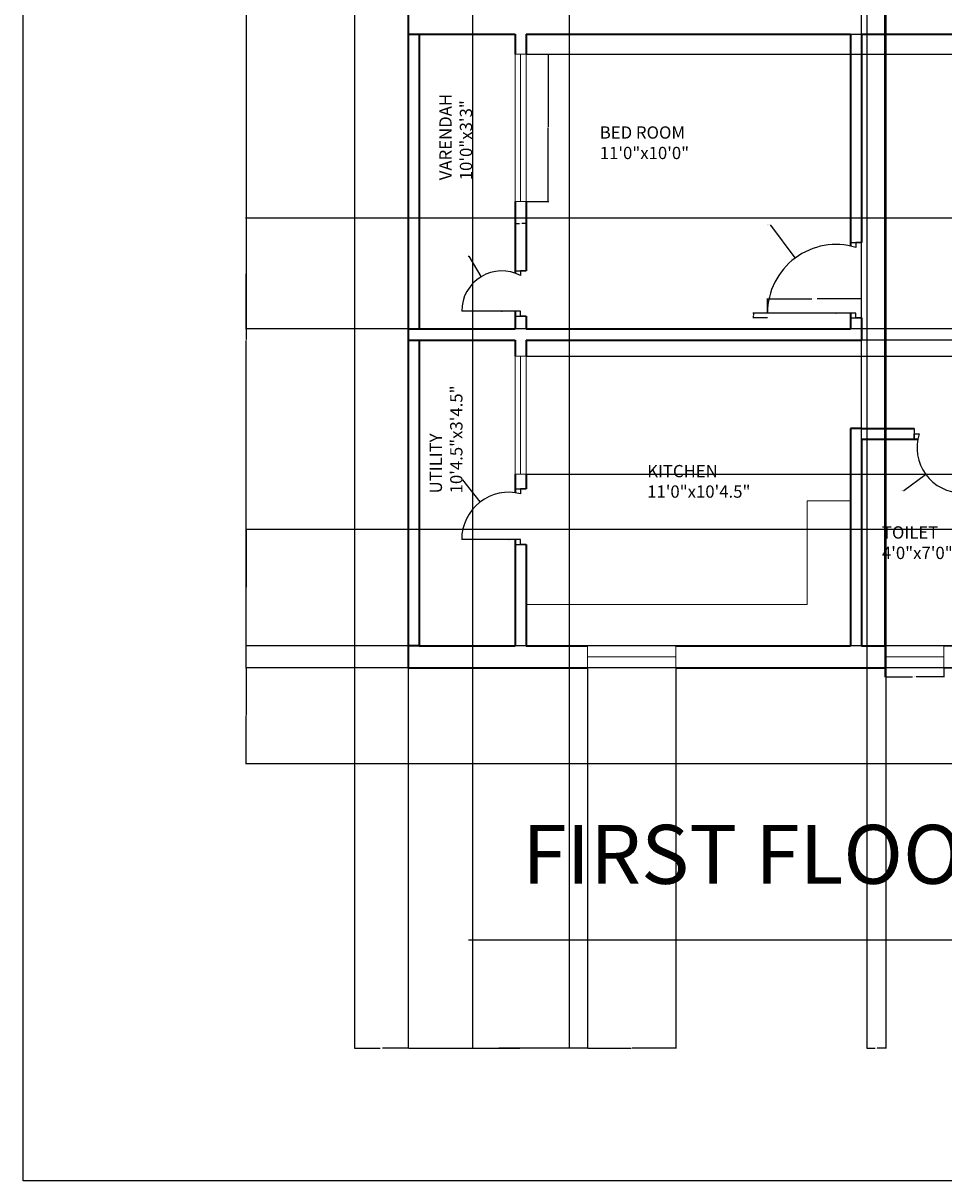
# Model space of a CAD drawing. Units: inches. Extents: x 1870 to 2611, y 1432 to 2511.
# Tile 1 of 5: x 1870 to 2245, y 1432 to 1903. Entities that reach past the tile are written whole.
import ezdxf

# ---------------------------------------------------------------- set-up
doc = ezdxf.new("R2010")
doc.units = ezdxf.units.IN
for name, color, linetype, lineweight in [('A-ANNO-DIMS', 2, 'Continuous', 18), ('A-ANNO-TTLB', 7, 'Continuous', 25), ('A-AREA-IDEN', 7, 'Continuous', 18), ('A-DOOR', 31, 'Continuous', 25), ('A-FLOR-FIXT', 8, 'Continuous', 18), ('A-GLAZ', 201, 'Continuous', 18), ('A-WALL', 7, 'Continuous', 35)]:
    doc.layers.add(name, color=color, linetype=linetype, lineweight=lineweight)
doc.styles.get("Standard").update_dxf_attribs({"font": 'arial.ttf'})
doc.dimstyles.get("Standard").update_dxf_attribs({"dimtxt": 0.18, "dimasz": 0.18, "dimexe": 0.18, "dimexo": 0.0625, "dimgap": 0.09, "dimtad": 0, "dimtih": 1, "dimtoh": 1, "dimdec": 4, "dimzin": 0, "dimdsep": 46, "dimtxsty": 'Standard', "dimcen": 0.09, "dimadec": 0, "dimazin": 0, "dimtfac": 1, "dimtdec": 4, "dimtofl": 0, "dimtmove": 0, "dimatfit": 3, "dimfxl": 1, "dimtolj": 1, "dimtzin": 0, "dimarcsym": 0})

# ---------------------------------------------------------------- blocks, each defined once
blk = doc.blocks.new('DOOR-LEAF-36-JAMB-4P5')
for p, q in [((36, 2), (0, 2)), ((33.75, 0), (38.25, 0)), ((36, 0), (36, 2)), ((38.25, 0), (36, 0))]:
    blk.add_line(p, q)
blk = doc.blocks.new('DOOR-LEAF-24-JAMB-4P5')
for p, q in [((2, 2.25), (2, 26.25)), ((0, 4.5), (0, 0)), ((0, 0), (0, 2.25)), ((0, 2.25), (2, 2.25))]:
    blk.add_line(p, q)
blk = doc.blocks.new('WIN-24-FRAME-9')
for p, q in [((0, 9), (0, 0)), ((24, 9), (0, 9)), ((24, 4.5), (24, 9)), ((24, 9), (24, 0)), ((0, 0), (0, 4.5)), ((0, 4.5), (24, 4.5)), ((0, 0), (24, 0))]:
    blk.add_line(p, q)
blk = doc.blocks.new('WIN-60-FRAME-4P5')
for p, q in [((0, 60), (4.5, 60)), ((0, 60), (0, 0)), ((4.5, 60), (2.25, 60)), ((2.25, 60), (2.25, 0)), ((4.5, 60), (4.5, 0)), ((2.25, 0), (0, 0)), ((0, 0), (4.5, 0))]:
    blk.add_line(p, q)
blk = doc.blocks.new('*D13')
at = {"layer": 'A-ANNO-DIMS', "color": 0, "lineweight": -2, "transparency": 16777216}
for p, q in [((2172.77, 1784.92), (2172.77, 1790.78)), ((2172.95, 1790.6), (2190.84, 1790.6)), ((2210.84, 1790.6), (2192.95, 1790.6)), ((2211.02, 1784.92), (2211.02, 1790.78))]:
    blk.add_line(p, q, dxfattribs=at)
at = {"layer": 'A-ANNO-DIMS', "color": 0, "transparency": 16777216}
for points in [[(2172.95, 1790.63), (2172.95, 1790.57), (2172.77, 1790.6)], [(2210.84, 1790.63), (2210.84, 1790.57), (2211.02, 1790.6)]]:
    blk.add_solid(points, dxfattribs=at)
at = {"layer": 'Defpoints', "color": 0, "transparency": 16777216}
for p in [(2211.02, 1790.6), (2172.77, 1784.86), (2211.02, 1784.86)]:
    blk.add_point(p, dxfattribs=at)
at = {"layer": 'A-ANNO-DIMS', "color": 0, "transparency": 16777216, "insert": (2191.89, 1790.6), "char_height": 0.18, "attachment_point": 5}
blk.add_mtext('\\A1;DOOR B 38 TYP.', dxfattribs=at)
blk = doc.blocks.new('*D14')
at = {"layer": 'A-ANNO-DIMS', "color": 0, "lineweight": -2, "transparency": 16777216}
for p, q in [((2172.71, 1784.86), (2166.85, 1784.86)), ((2172.71, 1782.86), (2166.85, 1782.86)), ((2167.03, 1784.68), (2167.03, 1784.04)), ((2167.03, 1783.04), (2167.03, 1783.68))]:
    blk.add_line(p, q, dxfattribs=at)
at = {"layer": 'A-ANNO-DIMS', "color": 0, "transparency": 16777216}
for points in [[(2167, 1784.68), (2167.06, 1784.68), (2167.03, 1784.86)], [(2167, 1783.04), (2167.06, 1783.04), (2167.03, 1782.86)]]:
    blk.add_solid(points, dxfattribs=at)
at = {"layer": 'Defpoints', "color": 0, "transparency": 16777216}
for p in [(2167.03, 1784.86), (2172.77, 1784.86), (2172.77, 1782.86)]:
    blk.add_point(p, dxfattribs=at)
at = {"layer": 'A-ANNO-DIMS', "color": 0, "transparency": 16777216, "insert": (2167.03, 1783.86), "char_height": 0.18, "attachment_point": 5}
blk.add_mtext('\\A1;2 TYP.', dxfattribs=at)
blk = doc.blocks.new('*D15')
at = {"layer": 'A-ANNO-DIMS', "color": 0, "lineweight": -2, "transparency": 16777216}
for p, q in [((2074.58, 1890.28), (2083.7, 1890.28)), ((2083.52, 1890.1), (2083.52, 1860.46)), ((2083.52, 1830.46), (2083.52, 1860.1)), ((2074.58, 1830.28), (2083.7, 1830.28))]:
    blk.add_line(p, q, dxfattribs=at)
at = {"layer": 'A-ANNO-DIMS', "color": 0, "transparency": 16777216}
for points in [[(2083.49, 1890.1), (2083.55, 1890.1), (2083.52, 1890.28)], [(2083.49, 1830.46), (2083.55, 1830.46), (2083.52, 1830.28)]]:
    blk.add_solid(points, dxfattribs=at)
at = {"layer": 'Defpoints', "color": 0, "transparency": 16777216}
for p in [(2074.52, 1890.28), (2074.52, 1830.28), (2083.52, 1830.28)]:
    blk.add_point(p, dxfattribs=at)
at = {"layer": 'A-ANNO-DIMS', "color": 0, "transparency": 16777216, "insert": (2083.52, 1860.28), "char_height": 0.18, "attachment_point": 5}
blk.add_mtext('\\A1;W2 60 TYP.', dxfattribs=at)
blk = doc.blocks.new('*D16')
at = {"layer": 'A-ANNO-DIMS', "color": 0, "lineweight": -2, "transparency": 16777216}
for p, q in [((2070.02, 1830.22), (2070.02, 1821.1)), ((2074.52, 1830.22), (2074.52, 1821.1)), ((2070.2, 1821.28), (2071.81, 1821.28)), ((2074.34, 1821.28), (2072.73, 1821.28))]:
    blk.add_line(p, q, dxfattribs=at)
at = {"layer": 'A-ANNO-DIMS', "color": 0, "transparency": 16777216}
for points in [[(2070.2, 1821.31), (2070.2, 1821.25), (2070.02, 1821.28)], [(2074.34, 1821.31), (2074.34, 1821.25), (2074.52, 1821.28)]]:
    blk.add_solid(points, dxfattribs=at)
at = {"layer": 'Defpoints', "color": 0, "transparency": 16777216}
for p in [(2070.02, 1830.28), (2074.52, 1830.28), (2070.02, 1821.28)]:
    blk.add_point(p, dxfattribs=at)
at = {"layer": 'A-ANNO-DIMS', "color": 0, "transparency": 16777216, "insert": (2072.27, 1821.28), "char_height": 0.18, "attachment_point": 5}
blk.add_mtext('\\A1;5 TYP.', dxfattribs=at)
blk = doc.blocks.new('*D17')
at = {"layer": 'A-ANNO-DIMS', "color": 0, "lineweight": -2, "transparency": 16777216}
for p, q in [((2220.56, 1640.3), (2220.56, 1636.59)), ((2244.56, 1640.3), (2244.56, 1636.59)), ((2220.74, 1636.77), (2231.8, 1636.77)), ((2244.38, 1636.77), (2233.31, 1636.77))]:
    blk.add_line(p, q, dxfattribs=at)
at = {"layer": 'A-ANNO-DIMS', "color": 0, "transparency": 16777216}
for points in [[(2220.74, 1636.8), (2220.74, 1636.74), (2220.56, 1636.77)], [(2244.38, 1636.8), (2244.38, 1636.74), (2244.56, 1636.77)]]:
    blk.add_solid(points, dxfattribs=at)
at = {"layer": 'Defpoints', "color": 0, "transparency": 16777216}
for p in [(2220.56, 1640.37), (2244.56, 1640.37), (2220.56, 1636.77)]:
    blk.add_point(p, dxfattribs=at)
at = {"layer": 'A-ANNO-DIMS', "color": 0, "transparency": 16777216, "insert": (2232.56, 1636.77), "char_height": 0.18, "attachment_point": 5}
blk.add_mtext('\\A1;W3 24 TYP.', dxfattribs=at)
blk = doc.blocks.new('*D18')
at = {"layer": 'A-ANNO-DIMS', "color": 0, "lineweight": -2, "transparency": 16777216}
for p, q in [((2244.62, 1649.37), (2248.34, 1649.37)), ((2248.16, 1649.19), (2248.16, 1645.05)), ((2244.62, 1640.37), (2248.34, 1640.37)), ((2248.16, 1640.55), (2248.16, 1644.69))]:
    blk.add_line(p, q, dxfattribs=at)
at = {"layer": 'A-ANNO-DIMS', "color": 0, "transparency": 16777216}
for points in [[(2248.13, 1649.19), (2248.19, 1649.19), (2248.16, 1649.37)], [(2248.13, 1640.55), (2248.19, 1640.55), (2248.16, 1640.37)]]:
    blk.add_solid(points, dxfattribs=at)
at = {"layer": 'Defpoints', "color": 0, "transparency": 16777216}
for p in [(2244.56, 1649.37), (2244.56, 1640.37), (2248.16, 1640.37)]:
    blk.add_point(p, dxfattribs=at)
at = {"layer": 'A-ANNO-DIMS', "color": 0, "transparency": 16777216, "insert": (2248.16, 1644.87), "char_height": 0.18, "attachment_point": 5}
blk.add_mtext('\\A1;9 TYP.', dxfattribs=at)
blk = doc.blocks.new('*D29')
at = {"layer": 'A-ANNO-DIMS', "color": 0, "lineweight": -2, "transparency": 16777216}
for p, q in [((2026.46, 1907.37), (1960.31, 1907.37)), ((1960.49, 1907.19), (1960.49, 1774.05)), ((1960.49, 1640.55), (1960.49, 1773.69)), ((2026.46, 1640.37), (1960.31, 1640.37))]:
    blk.add_line(p, q, dxfattribs=at)
at = {"layer": 'A-ANNO-DIMS', "color": 0, "transparency": 16777216}
for points in [[(1960.46, 1907.19), (1960.52, 1907.19), (1960.49, 1907.37)], [(1960.46, 1640.55), (1960.52, 1640.55), (1960.49, 1640.37)]]:
    blk.add_solid(points, dxfattribs=at)
at = {"layer": 'Defpoints', "color": 0, "transparency": 16777216}
for p in [(2026.52, 1907.37), (1960.49, 1640.37), (2026.52, 1640.37)]:
    blk.add_point(p, dxfattribs=at)
at = {"layer": 'A-ANNO-DIMS', "color": 0, "transparency": 16777216, "insert": (1960.49, 1773.87), "char_height": 0.18, "attachment_point": 5}
blk.add_mtext('\\A1;267', dxfattribs=at)
blk = doc.blocks.new('*D30')
at = {"layer": 'A-ANNO-DIMS', "color": 0, "lineweight": -2, "transparency": 16777216}
for p, q in [((2004.64, 2027.3), (2004.64, 1485.35)), ((2026.52, 2027.3), (2026.52, 1485.35)), ((2004.82, 1485.53), (2015.11, 1485.53)), ((2026.34, 1485.53), (2016.04, 1485.53))]:
    blk.add_line(p, q, dxfattribs=at)
at = {"layer": 'A-ANNO-DIMS', "color": 0, "transparency": 16777216}
for points in [[(2004.82, 1485.56), (2004.82, 1485.5), (2004.64, 1485.53)], [(2026.34, 1485.56), (2026.34, 1485.5), (2026.52, 1485.53)]]:
    blk.add_solid(points, dxfattribs=at)
at = {"layer": 'Defpoints', "color": 0, "transparency": 16777216}
for p in [(2004.64, 2027.37), (2026.52, 2027.37), (2026.52, 1485.53)]:
    blk.add_point(p, dxfattribs=at)
at = {"layer": 'A-ANNO-DIMS', "color": 0, "transparency": 16777216, "insert": (2015.58, 1485.53), "char_height": 0.18, "attachment_point": 5}
blk.add_mtext('\\A1;21.882', dxfattribs=at)
blk = doc.blocks.new('*D32')
at = {"layer": 'A-ANNO-DIMS', "color": 0, "lineweight": -2, "transparency": 16777216}
for p, q in [((2311.46, 1640.37), (1960.31, 1640.37)), ((1960.49, 1640.19), (1960.49, 1621.05)), ((1960.49, 1601.54), (1960.49, 1620.68)), ((2311.46, 1601.36), (1960.31, 1601.36))]:
    blk.add_line(p, q, dxfattribs=at)
at = {"layer": 'A-ANNO-DIMS', "color": 0, "transparency": 16777216}
for points in [[(1960.46, 1640.19), (1960.52, 1640.19), (1960.49, 1640.37)], [(1960.46, 1601.54), (1960.52, 1601.54), (1960.49, 1601.36)]]:
    blk.add_solid(points, dxfattribs=at)
at = {"layer": 'Defpoints', "color": 0, "transparency": 16777216}
for p in [(1960.49, 1640.37), (2311.52, 1640.37), (2311.52, 1601.36)]:
    blk.add_point(p, dxfattribs=at)
at = {"layer": 'A-ANNO-DIMS', "color": 0, "transparency": 16777216, "insert": (1960.49, 1620.86), "char_height": 0.18, "attachment_point": 5}
blk.add_mtext('\\A1;39.01', dxfattribs=at)
blk = doc.blocks.new('*D39')
at = {"layer": 'A-ANNO-DIMS', "color": 0, "lineweight": -2, "transparency": 16777216}
for p, q in [((2052.64, 2396.3), (2052.64, 1485.35)), ((2092.09, 2396.3), (2092.09, 1485.35)), ((2052.82, 1485.53), (2071.97, 1485.53)), ((2091.91, 1485.53), (2072.76, 1485.53))]:
    blk.add_line(p, q, dxfattribs=at)
at = {"layer": 'A-ANNO-DIMS', "color": 0, "transparency": 16777216}
for points in [[(2052.82, 1485.56), (2052.82, 1485.5), (2052.64, 1485.53)], [(2091.91, 1485.56), (2091.91, 1485.5), (2092.09, 1485.53)]]:
    blk.add_solid(points, dxfattribs=at)
at = {"layer": 'Defpoints', "color": 0, "transparency": 16777216}
for p in [(2052.64, 2396.37), (2092.09, 2396.37), (2092.09, 1485.53)]:
    blk.add_point(p, dxfattribs=at)
at = {"layer": 'A-ANNO-DIMS', "color": 0, "transparency": 16777216, "insert": (2072.36, 1485.53), "char_height": 0.18, "attachment_point": 5}
blk.add_mtext('\\A1;39.45', dxfattribs=at)
blk = doc.blocks.new('*D40')
at = {"layer": 'A-ANNO-DIMS', "color": 0, "lineweight": -2, "transparency": 16777216}
for p, q in [((2213.14, 2396.3), (2213.14, 1485.35)), ((2220.9, 2396.3), (2220.9, 1485.35)), ((2213.32, 1485.53), (2216.63, 1485.53)), ((2220.72, 1485.53), (2217.41, 1485.53))]:
    blk.add_line(p, q, dxfattribs=at)
at = {"layer": 'A-ANNO-DIMS', "color": 0, "transparency": 16777216}
for points in [[(2213.32, 1485.56), (2213.32, 1485.5), (2213.14, 1485.53)], [(2220.72, 1485.56), (2220.72, 1485.5), (2220.9, 1485.53)]]:
    blk.add_solid(points, dxfattribs=at)
at = {"layer": 'Defpoints', "color": 0, "transparency": 16777216}
for p in [(2213.14, 2396.37), (2220.9, 2396.37), (2220.9, 1485.53)]:
    blk.add_point(p, dxfattribs=at)
at = {"layer": 'A-ANNO-DIMS', "color": 0, "transparency": 16777216, "insert": (2217.02, 1485.53), "char_height": 0.18, "attachment_point": 5}
blk.add_mtext('\\A1;7.766', dxfattribs=at)
blk = doc.blocks.new('*D43')
at = {"layer": 'A-ANNO-DIMS', "color": 0, "lineweight": -2, "transparency": 16777216}
for p, q in [((2099.45, 1640.3), (2099.45, 1485.35)), ((2135.45, 1640.3), (2135.45, 1485.35)), ((2099.63, 1485.53), (2117.23, 1485.53)), ((2135.27, 1485.53), (2117.67, 1485.53))]:
    blk.add_line(p, q, dxfattribs=at)
at = {"layer": 'A-ANNO-DIMS', "color": 0, "transparency": 16777216}
for points in [[(2099.63, 1485.56), (2099.63, 1485.5), (2099.45, 1485.53)], [(2135.27, 1485.56), (2135.27, 1485.5), (2135.45, 1485.53)]]:
    blk.add_solid(points, dxfattribs=at)
at = {"layer": 'Defpoints', "color": 0, "transparency": 16777216}
for p in [(2099.45, 1640.37), (2135.45, 1640.37), (2135.45, 1485.53)]:
    blk.add_point(p, dxfattribs=at)
at = {"layer": 'A-ANNO-DIMS', "color": 0, "transparency": 16777216, "insert": (2117.45, 1485.53), "char_height": 0.18, "attachment_point": 5}
blk.add_mtext('\\A1;36', dxfattribs=at)
blk = doc.blocks.new('*D44')
at = {"layer": 'A-ANNO-DIMS', "color": 0, "lineweight": -2, "transparency": 16777216}
for p, q in [((2026.52, 1640.3), (2026.52, 1485.35)), ((2099.45, 1640.3), (2099.45, 1485.35)), ((2026.7, 1485.53), (2062.59, 1485.53)), ((2099.27, 1485.53), (2063.38, 1485.53))]:
    blk.add_line(p, q, dxfattribs=at)
at = {"layer": 'A-ANNO-DIMS', "color": 0, "transparency": 16777216}
for points in [[(2026.7, 1485.56), (2026.7, 1485.5), (2026.52, 1485.53)], [(2099.27, 1485.56), (2099.27, 1485.5), (2099.45, 1485.53)]]:
    blk.add_solid(points, dxfattribs=at)
at = {"layer": 'Defpoints', "color": 0, "transparency": 16777216}
for p in [(2026.52, 1640.37), (2099.45, 1640.37), (2099.45, 1485.53)]:
    blk.add_point(p, dxfattribs=at)
at = {"layer": 'A-ANNO-DIMS', "color": 0, "transparency": 16777216, "insert": (2062.99, 1485.53), "char_height": 0.18, "attachment_point": 5}
blk.add_mtext('\\A1;72.93', dxfattribs=at)
blk = doc.blocks.new('*D45')
at = {"layer": 'A-ANNO-DIMS', "color": 0, "lineweight": -2, "transparency": 16777216}
for p, q in [((2211.02, 1649.43), (2211.02, 2449.7)), ((2211.2, 2449.52), (2215.39, 2449.52)), ((2220.38, 2449.52), (2216.18, 2449.52)), ((2220.56, 1649.43), (2220.56, 2449.7))]:
    blk.add_line(p, q, dxfattribs=at)
at = {"layer": 'A-ANNO-DIMS', "color": 0, "transparency": 16777216}
for points in [[(2211.2, 2449.55), (2211.2, 2449.49), (2211.02, 2449.52)], [(2220.38, 2449.55), (2220.38, 2449.49), (2220.56, 2449.52)]]:
    blk.add_solid(points, dxfattribs=at)
at = {"layer": 'Defpoints', "color": 0, "transparency": 16777216}
for p in [(2220.56, 2449.52), (2211.02, 1649.37), (2220.56, 1649.37)]:
    blk.add_point(p, dxfattribs=at)
at = {"layer": 'A-ANNO-DIMS', "color": 0, "transparency": 16777216, "insert": (2215.79, 2449.52), "char_height": 0.18, "attachment_point": 5}
blk.add_mtext('\\A1;9.537', dxfattribs=at)
blk = doc.blocks.new('*D49')
at = {"layer": 'A-ANNO-DIMS', "color": 0, "lineweight": -2, "transparency": 16777216}
for p, q in [((2471.07, 1823.42), (1960.31, 1823.42)), ((1960.49, 1823.24), (1960.49, 1801.08)), ((1960.49, 1778.55), (1960.49, 1800.71)), ((2471.07, 1778.37), (1960.31, 1778.37))]:
    blk.add_line(p, q, dxfattribs=at)
at = {"layer": 'A-ANNO-DIMS', "color": 0, "transparency": 16777216}
for points in [[(1960.46, 1823.24), (1960.52, 1823.24), (1960.49, 1823.42)], [(1960.46, 1778.55), (1960.52, 1778.55), (1960.49, 1778.37)]]:
    blk.add_solid(points, dxfattribs=at)
at = {"layer": 'Defpoints', "color": 0, "transparency": 16777216}
for p in [(1960.49, 1823.42), (2471.14, 1823.42), (2471.14, 1778.37)]:
    blk.add_point(p, dxfattribs=at)
at = {"layer": 'A-ANNO-DIMS', "color": 0, "transparency": 16777216, "insert": (1960.49, 1800.89), "char_height": 0.18, "attachment_point": 5}
blk.add_mtext('\\A1;45.05', dxfattribs=at)
blk = doc.blocks.new('*D50')
at = {"layer": 'A-ANNO-DIMS', "color": 0, "lineweight": -2, "transparency": 16777216}
for p, q in [((2471.07, 1696.72), (1960.31, 1696.72)), ((1960.49, 1696.54), (1960.49, 1673.22)), ((1960.49, 1649.55), (1960.49, 1672.86)), ((2471.07, 1649.37), (1960.31, 1649.37))]:
    blk.add_line(p, q, dxfattribs=at)
at = {"layer": 'A-ANNO-DIMS', "color": 0, "transparency": 16777216}
for points in [[(1960.46, 1696.54), (1960.52, 1696.54), (1960.49, 1696.72)], [(1960.46, 1649.55), (1960.52, 1649.55), (1960.49, 1649.37)]]:
    blk.add_solid(points, dxfattribs=at)
at = {"layer": 'Defpoints', "color": 0, "transparency": 16777216}
for p in [(1960.49, 1696.72), (2471.14, 1696.72), (2471.14, 1649.37)]:
    blk.add_point(p, dxfattribs=at)
at = {"layer": 'A-ANNO-DIMS', "color": 0, "transparency": 16777216, "insert": (1960.49, 1673.04), "char_height": 0.18, "attachment_point": 5}
blk.add_mtext('\\A1;47.35', dxfattribs=at)
blk = doc.blocks.new('*D55')
at = {"layer": 'A-ANNO-DIMS', "color": 0, "lineweight": -2, "transparency": 16777216}
for p, q in [((2074.58, 1898.37), (2524.47, 1898.37)), ((2524.29, 1898.19), (2524.29, 1894.51)), ((2074.58, 1890.28), (2524.47, 1890.28)), ((2524.29, 1890.46), (2524.29, 1894.14))]:
    blk.add_line(p, q, dxfattribs=at)
at = {"layer": 'A-ANNO-DIMS', "color": 0, "transparency": 16777216}
for points in [[(2524.26, 1898.19), (2524.32, 1898.19), (2524.29, 1898.37)], [(2524.26, 1890.46), (2524.32, 1890.46), (2524.29, 1890.28)]]:
    blk.add_solid(points, dxfattribs=at)
at = {"layer": 'Defpoints', "color": 0, "transparency": 16777216}
for p in [(2074.52, 1898.37), (2524.29, 1898.37), (2074.52, 1890.28)]:
    blk.add_point(p, dxfattribs=at)
at = {"layer": 'A-ANNO-DIMS', "color": 0, "transparency": 16777216, "insert": (2524.29, 1894.32), "char_height": 0.18, "attachment_point": 5}
blk.add_mtext('\\A1;8.085', dxfattribs=at)
blk = doc.blocks.new('*D56')
at = {"layer": 'A-ANNO-DIMS', "color": 0, "lineweight": -2, "transparency": 16777216}
for p, q in [((2074.58, 1767.26), (2524.47, 1767.26)), ((2524.29, 1767.08), (2524.29, 1743.44)), ((2524.29, 1719.44), (2524.29, 1743.08)), ((2074.58, 1719.26), (2524.47, 1719.26))]:
    blk.add_line(p, q, dxfattribs=at)
at = {"layer": 'A-ANNO-DIMS', "color": 0, "transparency": 16777216}
for points in [[(2524.26, 1767.08), (2524.32, 1767.08), (2524.29, 1767.26)], [(2524.26, 1719.44), (2524.32, 1719.44), (2524.29, 1719.26)]]:
    blk.add_solid(points, dxfattribs=at)
at = {"layer": 'Defpoints', "color": 0, "transparency": 16777216}
for p in [(2074.52, 1767.26), (2524.29, 1767.26), (2074.52, 1719.26)]:
    blk.add_point(p, dxfattribs=at)
at = {"layer": 'A-ANNO-DIMS', "color": 0, "transparency": 16777216, "insert": (2524.29, 1743.26), "char_height": 0.18, "attachment_point": 5}
blk.add_mtext('\\A1;48', dxfattribs=at)
blk = doc.blocks.new('*D57')
at = {"layer": 'A-ANNO-DIMS', "color": 0, "lineweight": -2, "transparency": 16777216}
for p, q in [((2074.58, 1773.87), (2524.47, 1773.87)), ((2524.29, 1773.69), (2524.29, 1770.74)), ((2524.29, 1767.44), (2524.29, 1770.38)), ((2074.58, 1767.26), (2524.47, 1767.26))]:
    blk.add_line(p, q, dxfattribs=at)
at = {"layer": 'A-ANNO-DIMS', "color": 0, "transparency": 16777216}
for points in [[(2524.26, 1773.69), (2524.32, 1773.69), (2524.29, 1773.87)], [(2524.26, 1767.44), (2524.32, 1767.44), (2524.29, 1767.26)]]:
    blk.add_solid(points, dxfattribs=at)
at = {"layer": 'Defpoints', "color": 0, "transparency": 16777216}
for p in [(2074.52, 1773.87), (2524.29, 1773.87), (2074.52, 1767.26)]:
    blk.add_point(p, dxfattribs=at)
at = {"layer": 'A-ANNO-DIMS', "color": 0, "transparency": 16777216, "insert": (2524.29, 1770.56), "char_height": 0.18, "attachment_point": 5}
blk.add_mtext('\\A1;6.61', dxfattribs=at)
blk = doc.blocks.new('*D63')
at = {"layer": 'A-ANNO-DIMS', "color": 0, "lineweight": -2, "transparency": 16777216}
for p, q in [((2173.86, 1820.67), (2174.04, 1820.67)), ((2174.04, 1820.67), (2183.91, 1807.38)), ((2200.57, 1784.86), (2200.75, 1784.86)), ((2200.66, 1784.77), (2200.66, 1784.95))]:
    blk.add_line(p, q, dxfattribs=at)
at = {"layer": 'A-ANNO-DIMS', "color": 0, "transparency": 16777216}
blk.add_solid([(2183.94, 1807.4), (2183.89, 1807.37), (2184.02, 1807.24)], dxfattribs=at)
at = {"layer": 'Defpoints', "color": 0, "transparency": 16777216}
for p in [(2184.02, 1807.24), (2200.66, 1784.86)]:
    blk.add_point(p, dxfattribs=at)
at = {"layer": 'A-ANNO-DIMS', "color": 0, "transparency": 16777216, "insert": (2173.31, 1820.67), "char_height": 0.18, "attachment_point": 5}
blk.add_mtext('\\A1;R27.887', dxfattribs=at)
blk = doc.blocks.new('*D71')
at = {"layer": 'A-ANNO-DIMS', "color": 0, "lineweight": -2, "transparency": 16777216}
for p, q in [((2048.44, 1716.94), (2048.62, 1716.94)), ((2048.62, 1716.94), (2055.59, 1707.96)), ((2067.43, 1692.62), (2067.61, 1692.62)), ((2067.52, 1692.53), (2067.52, 1692.71))]:
    blk.add_line(p, q, dxfattribs=at)
at = {"layer": 'A-ANNO-DIMS', "color": 0, "transparency": 16777216}
blk.add_solid([(2055.62, 1707.98), (2055.57, 1707.94), (2055.7, 1707.82)], dxfattribs=at)
at = {"layer": 'Defpoints', "color": 0, "transparency": 16777216}
for p in [(2055.7, 1707.82), (2067.52, 1692.62)]:
    blk.add_point(p, dxfattribs=at)
at = {"layer": 'A-ANNO-DIMS', "color": 0, "transparency": 16777216, "insert": (2047.89, 1716.94), "char_height": 0.18, "attachment_point": 5}
blk.add_mtext('\\A1;R19.247', dxfattribs=at)
blk = doc.blocks.new('*D74')
at = {"layer": 'A-ANNO-DIMS', "color": 0, "lineweight": -2, "transparency": 16777216}
for p, q in [((2251.93, 1730.01), (2252.11, 1730.01)), ((2252.02, 1729.92), (2252.02, 1730.1)), ((2228.25, 1712.66), (2237.02, 1719.06)), ((2228.07, 1712.66), (2228.25, 1712.66))]:
    blk.add_line(p, q, dxfattribs=at)
at = {"layer": 'A-ANNO-DIMS', "color": 0, "transparency": 16777216}
blk.add_solid([(2237, 1719.08), (2237.04, 1719.04), (2237.17, 1719.17)], dxfattribs=at)
at = {"layer": 'Defpoints', "color": 0, "transparency": 16777216}
for p in [(2252.02, 1730.01), (2237.17, 1719.17)]:
    blk.add_point(p, dxfattribs=at)
at = {"layer": 'A-ANNO-DIMS', "color": 0, "transparency": 16777216, "insert": (2227.59, 1712.66), "char_height": 0.18, "attachment_point": 5}
blk.add_mtext('\\A1;R18.39', dxfattribs=at)
blk = doc.blocks.new('*D77')
at = {"layer": 'A-ANNO-DIMS', "color": 0, "lineweight": -2, "transparency": 16777216}
for p, q in [((2050.94, 1808.03), (2051.12, 1808.03)), ((2051.12, 1808.03), (2056.09, 1799.78)), ((2064.54, 1785.61), (2064.72, 1785.61)), ((2064.63, 1785.52), (2064.63, 1785.7))]:
    blk.add_line(p, q, dxfattribs=at)
at = {"layer": 'A-ANNO-DIMS', "color": 0, "transparency": 16777216}
blk.add_solid([(2056.12, 1799.79), (2056.06, 1799.76), (2056.18, 1799.63)], dxfattribs=at)
at = {"layer": 'Defpoints', "color": 0, "transparency": 16777216}
for p in [(2056.18, 1799.63), (2064.63, 1785.61)]:
    blk.add_point(p, dxfattribs=at)
at = {"layer": 'A-ANNO-DIMS', "color": 0, "transparency": 16777216, "insert": (2050.39, 1808.03), "char_height": 0.18, "attachment_point": 5}
blk.add_mtext('\\A1;R16.358', dxfattribs=at)

msp = doc.modelspace()

# ---------------------------------------------------------------- linework, layer by layer
at = {"layer": 'A-ANNO-TTLB'}
msp.add_line((2050.9784, 1529.6813), (2406.6559, 1529.6813), dxfattribs=at)
msp.add_lwpolyline([(1869.7418, 2510.8018), (2611.0646, 2510.8018), (2611.0646, 1431.531), (1869.7418, 1431.531)], close=True, dxfattribs=at)
at = {"layer": 'A-DOOR'}
for p, q in [((2206.5182, 1813.5628), (2208.6922, 1813.5628)), ((2208.6922, 1813.5628), (2208.6922, 1813.5628)), ((2208.6922, 1813.5628), (2211.0182, 1813.5628)), ((2211.0182, 1813.5628), (2208.6922, 1813.5628)), ((2208.6922, 1813.5628), (2208.6922, 1811.5628)), ((2070.0182, 1802.0777), (2074.5182, 1802.0777)), ((2074.5182, 1802.0777), (2072.2682, 1802.0777)), ((2072.2682, 1802.0777), (2072.2682, 1800.0777)), ((2206.5182, 1773.8669), (2206.5182, 1773.8669)), ((2232.5091, 1737.8669), (2232.5091, 1733.3669)), ((2232.5091, 1733.3669), (2232.5091, 1735.6169)), ((2232.5091, 1735.6169), (2234.5091, 1735.6169)), ((2070.0182, 1713.2727), (2074.5182, 1713.2727)), ((2074.5182, 1713.2727), (2072.2682, 1713.2727)), ((2072.2682, 1713.2727), (2072.2682, 1711.2727)), ((2074.5182, 1690.6217), (2074.5182, 1690.6217))]:
    msp.add_line(p, q, dxfattribs=at)
for centre, radius, start, end in [((2200.6553, 1784.8589), 27.8871, 73.250156, 180), ((2064.6262, 1785.6145), 16.358, 62.149119, 180), ((2252.0217, 1730.0064), 18.3894, 162.235951, 270), ((2067.5153, 1692.6217), 19.247, 75.703145, 180)]:
    msp.add_arc(centre, radius, start, end, dxfattribs=at)
at = {"layer": 'A-FLOR-FIXT'}
for p, q in [((2188.9261, 1666.2385), (2188.9261, 1708.3542)), ((2188.9261, 1708.3542), (2206.5182, 1708.3542)), ((2074.5182, 1666.2385), (2188.9261, 1666.2385))]:
    msp.add_line(p, q, dxfattribs=at)
at = {"layer": 'A-GLAZ'}
for p, q in [((2070.0182, 1890.2819), (2070.0182, 1890.2819)), ((2074.5182, 1890.2819), (2074.5182, 1890.2819)), ((2070.0182, 1767.257), (2074.5182, 1767.257)), ((2070.0182, 1767.257), (2070.0182, 1719.257)), ((2074.5182, 1767.257), (2072.2682, 1767.257)), ((2072.2682, 1767.257), (2072.2682, 1719.257)), ((2074.5182, 1767.257), (2074.5182, 1719.257)), ((2072.2682, 1719.257), (2070.0182, 1719.257)), ((2070.0182, 1719.257), (2074.5182, 1719.257)), ((2099.4519, 1649.3669), (2099.4519, 1640.3669)), ((2099.4519, 1649.3669), (2135.4519, 1649.3669)), ((2135.4519, 1644.8669), (2135.4519, 1649.3669)), ((2135.4519, 1649.3669), (2135.4519, 1640.3669)), ((2099.4519, 1640.3669), (2099.4519, 1644.8669)), ((2099.4519, 1644.8669), (2135.4519, 1644.8669)), ((2135.4519, 1640.3669), (2099.4519, 1640.3669))]:
    msp.add_line(p, q, dxfattribs=at)
at = {"layer": 'A-WALL'}
for p, q in [((2026.5182, 2027.3669), (2026.5182, 1640.3669)), ((2026.5182, 1898.3669), (2070.0182, 1898.3669)), ((2031.0182, 1898.3669), (2031.0182, 1778.3669)), ((2070.0182, 1898.3669), (2070.0182, 1890.2819)), ((2074.5182, 1898.3669), (2074.5182, 1890.2819)), ((2074.5182, 1898.3669), (2206.5182, 1898.3669)), ((2206.5182, 1898.3669), (2206.5182, 1812.1227)), ((2211.0182, 1898.3669), (2211.0182, 1813.5628)), ((2211.0182, 1898.3669), (2331.8969, 1898.3669)), ((2070.0182, 1830.2819), (2070.0182, 1801.0582)), ((2074.5182, 1830.2819), (2074.5182, 1802.0777)), ((2070.0182, 1785.6145), (2070.0182, 1778.3669)), ((2074.5182, 1783.6145), (2074.5182, 1778.3669)), ((2206.5182, 1784.8589), (2206.5182, 1778.3669)), ((2211.0182, 1782.8589), (2211.0182, 1778.3669)), ((2026.5182, 1778.3669), (2070.0182, 1778.3669)), ((2074.5182, 1778.3669), (2206.5182, 1778.3669)), ((2211.0182, 1778.3669), (2211.0182, 1773.8669)), ((2026.5182, 1773.8669), (2070.0182, 1773.8669)), ((2031.0182, 1773.8669), (2031.0182, 1649.3669)), ((2070.0182, 1773.8669), (2070.0182, 1767.257)), ((2074.5182, 1773.8669), (2206.5182, 1773.8669)), ((2074.5182, 1773.8669), (2074.5182, 1767.257)), ((2206.5182, 1773.8669), (2211.0182, 1773.8669)), ((2206.5182, 1737.8669), (2206.5182, 1649.3669)), ((2211.0182, 1737.8669), (2206.5182, 1737.8669)), ((2206.5182, 1737.8669), (2206.5182, 1737.8669)), ((2211.0182, 1737.8669), (2232.5091, 1737.8669)), ((2211.0182, 1733.3669), (2211.0182, 1649.3669)), ((2233.942, 1733.3669), (2211.0182, 1733.3669)), ((2070.0182, 1719.257), (2070.0182, 1711.7053)), ((2074.5182, 1719.257), (2074.5182, 1713.2727)), ((2070.0182, 1692.6217), (2070.0182, 1649.3669)), ((2074.5182, 1690.6217), (2074.5182, 1649.3669)), ((2031.0182, 1649.3669), (2026.5182, 1649.3669)), ((2031.0182, 1649.3669), (2070.0182, 1649.3669)), ((2074.5182, 1649.3669), (2099.4519, 1649.3669)), ((2135.4519, 1649.3669), (2206.5182, 1649.3669)), ((2211.0182, 1649.3669), (2220.5557, 1649.3669)), ((2026.5182, 1640.3669), (2099.4519, 1640.3669)), ((2135.4519, 1640.3669), (2220.5557, 1640.3669))]:
    msp.add_line(p, q, dxfattribs=at)

# ---------------------------------------------------------------- block references
at = {"layer": 'A-DOOR'}
for p, rotation in [((2074.5182, 1783.6142), 89.99999999999935), ((2074.5182, 1690.6214), 89.99999999999991)]:
    msp.add_blockref('DOOR-LEAF-24-JAMB-4P5', p, dxfattribs=dict(at, rotation=rotation))
msp.add_blockref('DOOR-LEAF-36-JAMB-4P5', (2172.7683, 1782.8588), dxfattribs=at)
at = {"layer": 'A-GLAZ', "rotation": 180}
for name, p in [('WIN-60-FRAME-4P5', (2074.5182, 1890.2818)), ('WIN-24-FRAME-9', (2244.5555, 1649.3669))]:
    msp.add_blockref(name, p, dxfattribs=at)

# ---------------------------------------------------------------- texts
at = {"layer": 'A-ANNO-TTLB', "insert": (2072.8808, 1576.4623), "char_height": 24, "attachment_point": 1}
msp.add_mtext_dynamic_manual_height_columns('FIRST FLOOR PLAN', width=470.964305, gutter_width=12.5, heights=[0], dxfattribs=at)
at = {"layer": 'A-AREA-IDEN', "char_height": 5, "attachment_point": 1, "rotation": 90}
for s, width, insert in [('VARENDAH\\P10\'0"x3\'3"', 43.074536, (2039.1939, 1838.9092)), ('UTILITY\\P10\'4.5"x3\'4.5"', 109.69956, (2035.2449, 1711.4208))]:
    msp.add_mtext_dynamic_manual_height_columns(s, width=width, gutter_width=12.5, heights=[0], dxfattribs=dict(at, insert=insert))
at = {"layer": 'A-AREA-IDEN', "char_height": 5, "attachment_point": 1}
for s, width, insert in [('BED ROOM\\P11\'0"x10\'0"', 102.036166, (2104.4821, 1860.8451)), ('KITCHEN\\P11\'0"x10\'4.5"', 111.440738, (2123.7704, 1722.9911)), ('TOILET\\P4\'0"x7\'0"', 39.670567, (2219.3477, 1698.0164))]:
    msp.add_mtext_dynamic_manual_height_columns(s, width=width, gutter_width=12.5, heights=[0], dxfattribs=dict(at, insert=insert))

# ---------------------------------------------------------------- dimensions: what is measured, and where the dimension line sits
at = {"layer": 'A-ANNO-DIMS'}
for base, p1, p2, override, picture, middle in [((2220.55567, 2449.51694), (2211.01824, 1649.36694), (2220.55567, 1649.36694), {"dimdec": 3, "dimlfac": 1, "dimrnd": 0, "dimzin": 0, "dimdsep": 46, "dimlunit": 2}, '*D45', (2215.78695, 2449.51694)), ((2092.0868, 1485.5313), (2052.6359, 2396.3669), (2092.0868, 2396.3669), {"dimdec": 2, "dimlfac": 1, "dimrnd": 0, "dimzin": 0, "dimdsep": 46, "dimlunit": 2}, '*D39', (2072.3614, 1485.5313)), ((2220.9018, 1485.5313), (2213.1359, 2396.3669), (2220.9018, 2396.3669), {"dimdec": 3, "dimlfac": 1, "dimrnd": 0, "dimzin": 0, "dimdsep": 46, "dimlunit": 2}, '*D40', (2217.0189, 1485.5313)), ((2026.5182, 1485.5313), (2004.6359, 2027.3669), (2026.5182, 2027.3669), {"dimdec": 3, "dimlfac": 1, "dimrnd": 0, "dimzin": 0, "dimdsep": 46, "dimlunit": 2}, '*D30', (2015.5771, 1485.5313)), ((2099.4519, 1485.5313), (2026.5182, 1640.3669), (2099.4519, 1640.3669), {"dimdec": 2, "dimlfac": 1, "dimrnd": 0, "dimzin": 0, "dimdsep": 46, "dimlunit": 2}, '*D44', (2062.9851, 1485.5313)), ((2135.4519, 1485.5313), (2099.4519, 1640.3669), (2135.4519, 1640.3669), {"dimdec": 0, "dimlfac": 1, "dimrnd": 0, "dimzin": 0, "dimdsep": 46, "dimlunit": 2}, '*D43', (2117.4519, 1485.5313))]:
    dim = msp.add_linear_dim(base=base, p1=p1, p2=p2, dimstyle='Standard', override=override, dxfattribs=at)
    dim.commit()
    dim.dimension.update_dxf_attribs({"geometry": picture, "text_midpoint": middle})
for base, p1, p2, override, picture, middle in [((1960.4859, 1640.3669), (2026.5182, 1907.3669), (2026.5182, 1640.3669), {"dimdec": 0, "dimlfac": 1, "dimrnd": 0, "dimzin": 0, "dimdsep": 46, "dimlunit": 2}, '*D29', (1960.4859, 1773.8669)), ((2524.2859, 1898.3669), (2074.5182, 1890.2819), (2074.5182, 1898.3669), {"dimdec": 3, "dimlfac": 1, "dimrnd": 0, "dimzin": 0, "dimdsep": 46, "dimlunit": 2}, '*D55', (2524.2859, 1894.3244)), ((1960.4859, 1823.4206), (2471.1359, 1778.3669), (2471.1359, 1823.4206), {"dimdec": 2, "dimlfac": 1, "dimrnd": 0, "dimzin": 0, "dimdsep": 46, "dimlunit": 2}, '*D49', (1960.4859, 1800.8937)), ((2524.2859, 1773.8669), (2074.5182, 1767.257), (2074.5182, 1773.8669), {"dimdec": 2, "dimlfac": 1, "dimrnd": 0, "dimzin": 0, "dimdsep": 46, "dimlunit": 2}, '*D57', (2524.2859, 1770.562)), ((2524.2859, 1767.257), (2074.5182, 1719.257), (2074.5182, 1767.257), {"dimdec": 0, "dimlfac": 1, "dimrnd": 0, "dimzin": 0, "dimdsep": 46, "dimlunit": 2}, '*D56', (2524.2859, 1743.257)), ((1960.4859, 1696.7177), (2471.1359, 1649.3669), (2471.1359, 1696.7177), {"dimdec": 2, "dimlfac": 1, "dimrnd": 0, "dimzin": 0, "dimdsep": 46, "dimlunit": 2}, '*D50', (1960.4859, 1673.0423)), ((1960.4859, 1640.3669), (2311.5182, 1601.3597), (2311.5182, 1640.3669), {"dimdec": 2, "dimlfac": 1, "dimrnd": 0, "dimzin": 0, "dimdsep": 46, "dimlunit": 2}, '*D32', (1960.4859, 1620.8633))]:
    dim = msp.add_linear_dim(base=base, p1=p1, p2=p2, angle=90, dimstyle='Standard', override=override, dxfattribs=at)
    dim.commit()
    dim.dimension.update_dxf_attribs({"geometry": picture, "text_midpoint": middle})
for base, p1, p2, angle, text, picture, middle in [((2083.5182, 1830.2819), (2074.5182, 1890.2819), (2074.5182, 1830.2819), 270, 'W2 <> TYP.', '*D15', (2083.5182, 1860.2819)), ((2070.0182391875, 1821.2818631396), (2074.5182391875, 1830.2818631396), (2070.0182391875, 1830.2818631396), 180, '<> TYP.', '*D16', (2072.2682391875, 1821.2818631396)), ((2167.0307, 1784.8589), (2172.7682, 1782.8589), (2172.7682, 1784.8589), 90, '<> TYP.', '*D14', (2167.0307, 1783.8589)), ((2248.1557, 1640.3669), (2244.5557, 1649.3669), (2244.5557, 1640.3669), 270, '<> TYP.', '*D18', (2248.1557, 1644.8669)), ((2220.5557, 1636.7669), (2244.5557, 1640.3669), (2220.5557, 1640.3669), 180, 'W3 <> TYP.', '*D17', (2232.5557, 1636.7669))]:
    dim = msp.add_linear_dim(base=base, p1=p1, p2=p2, angle=angle, text=text, dimstyle='Standard', override={"dimdec": 0, "dimlfac": 1, "dimrnd": 0, "dimzin": 0, "dimdsep": 46, "dimlunit": 2}, dxfattribs=at)
    dim.commit()
    dim.dimension.update_dxf_attribs({"geometry": picture, "text_midpoint": middle})
for center, mpoint, override, picture, middle in [((2200.6553, 1784.8589), (2184.0189, 1807.2401), {"dimdec": 3, "dimlfac": 1, "dimrnd": 0, "dimzin": 0, "dimdsep": 46, "dimlunit": 2}, '*D63', (2173.3073, 1820.6688)), ((2064.6262, 1785.6145), (2056.183, 1799.625), {"dimdec": 3, "dimlfac": 1, "dimrnd": 0, "dimzin": 0, "dimdsep": 46, "dimlunit": 2}, '*D77', (2050.3871, 1808.0313)), ((2252.0217, 1730.0064), (2237.1666, 1719.1667), {"dimdec": 2, "dimlfac": 1, "dimrnd": 0, "dimzin": 0, "dimdsep": 46, "dimlunit": 2}, '*D74', (2227.5936, 1712.663)), ((2067.5153, 1692.6217), (2055.7049, 1707.8192), {"dimdec": 3, "dimlfac": 1, "dimrnd": 0, "dimzin": 0, "dimdsep": 46, "dimlunit": 2}, '*D71', (2047.8889, 1716.9376))]:
    dim = msp.add_radius_dim(center=center, mpoint=mpoint, dimstyle='Standard', override=override, dxfattribs=at)
    dim.commit()
    dim.dimension.update_dxf_attribs({"geometry": picture, "text_midpoint": middle, "dimtype": 164})
dim = msp.add_linear_dim(base=(2211.0182, 1790.5964), p1=(2172.7682, 1784.8589), p2=(2211.0182, 1784.8589), text='DOOR B <> TYP.', dimstyle='Standard', override={"dimdec": 0, "dimlfac": 1, "dimrnd": 0, "dimzin": 0, "dimdsep": 46, "dimlunit": 2}, dxfattribs=at)
dim.commit()
dim.dimension.update_dxf_attribs({"geometry": '*D13', "text_midpoint": (2191.8932, 1790.5964)})

doc.saveas('drawing.dxf')
